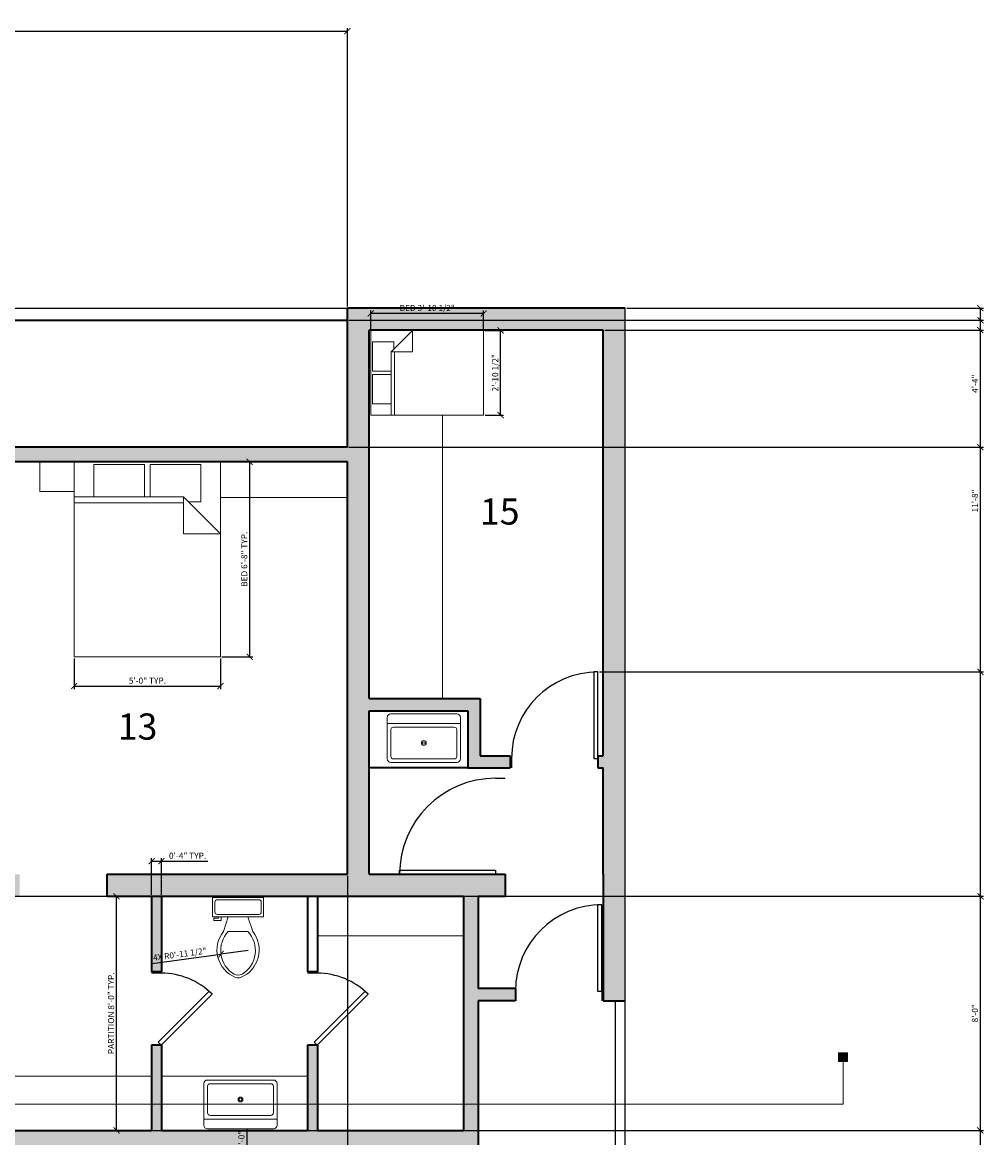
# Model space of a CAD drawing. Units: inches. Extents: x 3122 to 5933, y 1474 to 2995.
# Tile 12 of 12: x 5538 to 5932, y 2536 to 2993. Entities that reach past the tile are written whole.
import ezdxf

# ---------------------------------------------------------------- set-up
doc = ezdxf.new("R2010")
doc.units = ezdxf.units.IN
for name, color, linetype, lineweight in [('A-ANNO-DIMS', 2, 'Continuous', 18), ('A-ANNO-SYMB', 6, 'Continuous', 18), ('A-AREA-IDEN', 7, 'Continuous', 20), ('A-DOOR', 4, 'Continuous', 25), ('A-FLOR-CASE', 8, 'Continuous', 18), ('A-FLOR-FIXT', 9, 'Continuous', 18), ('A-FURN', 8, 'Continuous', 18), ('A-WALL', 7, 'Continuous', 35), ('A-WALL-PATT', 7, 'Continuous', 13), ('C-PROP', 7, 'Continuous', 25)]:
    doc.layers.add(name, color=color, linetype=linetype, lineweight=lineweight)
doc.styles.get("Standard").update_dxf_attribs({"font": 'arial.ttf'})
doc.dimstyles.new('ISO-25', dxfattribs={"dimtxt": 2.5, "dimasz": 2.5, "dimexe": 1.25, "dimexo": 0.625, "dimtad": 1, "dimdec": 0, "dimlunit": 3, "dimtxsty": 'Standard', "dimblk": 'ARCHTICK', "dimcen": 2.5, "dimadec": 0, "dimazin": 0, "dimtfac": 1, "dimtdec": 0, "dimtmove": 0, "dimatfit": 3, "dimfxl": 1, "dimarcsym": 0})

# ---------------------------------------------------------------- blocks, each defined once
blk = doc.blocks.new('*U28')
for p, q in [((0, 0), (0, -100)), ((-900, 0), (-900, -100))]:
    blk.add_line(p, q)
blk.add_lwpolyline([(0, 0), (0, 900), (-43.75, 900), (-43.75, 0)], close=True)
blk.add_arc((0, 0), 900, 90, 180)
blk = doc.blocks.new('*U29')
for p, q in [((0, 0), (0, 100)), ((750, 0), (750, 100))]:
    blk.add_line(p, q)
blk.add_lwpolyline([(0, 0), (530, -530), (561, -499), (31, 31)], close=True)
blk.add_arc((0, 0), 750, 315, 0)
blk = doc.blocks.new('*U30')
for p, q in [((0, 0), (0, -100)), ((1000, 0), (1000, -100))]:
    blk.add_line(p, q)
blk.add_lwpolyline([(0, 0), (0, 1000), (43.75, 1000), (43.75, 0)], close=True)
blk.add_arc((0, 0), 1000, 0, 90)
blk = doc.blocks.new('Bed - Queen')
for p, q in [((0, -80.00003), (0, 0)), ((0, 0), (59.99999, 0)), ((59.99999, 0), (59.99999, -80.00003)), ((7.99999, -1.2), (28.79998, -1.2)), ((7.99999, -14.4), (7.99999, -1.2)), ((28.79998, -1.2), (28.79998, -14.4)), ((31.19999, -1.2), (51.99999, -1.2)), ((31.19999, -14.4), (31.19999, -1.2)), ((51.99999, -1.2), (51.99999, -16.4)), ((0, -14.4), (44.8, -14.4)), ((44.8, -16.8), (0, -16.8)), ((59.99999, -29.6), (44.8, -14.4)), ((44.8, -14.4), (44.8, -29.6)), ((51.99999, -16.4), (46.79936, -16.4)), ((44.8, -29.6), (59.99999, -29.6)), ((59.99999, -80.00003), (0, -80.00003))]:
    blk.add_line(p, q)
blk = doc.blocks.new('Sink-single - 30 in top')
blk.add_line((-15, -3.999996), (15, -3.999996))
for points in [[(-13.5, 0), (13.5, 0)], [(-15, -18.499996), (-15, -1.5)], [(15, -1.5), (15, -18.499996)], [(-13.5, -17.499996), (-13.5, -6.499996)], [(-12.5, -5.499996), (12.5, -5.499996)], [(13.5, -6.499996), (13.5, -17.499996)], [(13.5, -19.999996), (-13.5, -19.999996)], [(12.5, -18.499996), (-12.5, -18.499996)]]:
    blk.add_lwpolyline(points)
for radius in [1, 0.5]:
    blk.add_circle((0, -11.999996), radius)
for centre, radius, start, end in [((-13.5, -1.5), 1.5, 90, 180), ((13.5, -1.5), 1.5, 0, 90), ((-12.5, -6.499996), 1, 90, 180), ((12.5, -6.499996), 1, 0, 90), ((-12.5, -17.499996), 1, 180, 270), ((12.5, -17.499996), 1, 270, 0), ((-13.5, -18.499996), 1.5, 180, 270), ((13.5, -18.499996), 1.5, 270, 0)]:
    blk.add_arc(centre, radius, start, end)
blk = doc.blocks.new('Toilet - top')
for p, q in [((9.5, -6), (9.5, -2)), ((-10, -8.5), (-8, -8.5)), ((-10, -9.5), (-10, -8.5)), ((-8, -8.5), (-8, -8)), ((-7, -8), (-7, -9.5)), ((-4, -8), (-6, -14)), ((4, -8), (6, -14)), ((-7, -9.5), (-10, -9.5)), ((4, -14), (-4, -14))]:
    blk.add_line(p, q)
blk.add_lwpolyline([(10.5, -8), (10.5, 0), (-10.5, 0), (-10.5, -8)], close=True)
for points in [[(-9.5, -2), (-9.5, -6)], [(8.5, -1), (-8.5, -1)], [(-8.5, -7), (8.5, -7)]]:
    blk.add_lwpolyline(points)
for centre, radius, start, end in [((-8.62, -1.88), 0.884, 81.8699, 188.1301), ((8.62, -1.88), 0.884, 351.8699, 98.1301), ((-8.62, -6.12), 0.884, 171.8699, 278.1301), ((8.62, -6.12), 0.884, 261.8699, 8.1301), ((3.52, -21.58), 12.17, 141.4691, 247.9714), ((4.2, -21.82), 11.33, 136.3677, 238.9468), ((-3.52, -21.58), 12.17, 292.0284, 38.5307), ((-4.2, -21.82), 11.33, 301.053, 43.6321), ((0, -27.88), 4, 245.7318, 294.2682), ((0, -29), 4, 254.8605, 285.1395)]:
    blk.add_arc(centre, radius, start, end)
blk = doc.blocks.new('SECTION-LINE-END-MARK')
h = blk.add_hatch(color=256)
h.dxf.hatch_style = 1
h.paths.add_polyline_path([(3.68, 3.54), (0, 3.54), (0, 0), (3.68, 0)])
blk.add_lwpolyline([(0, 3.54), (3.68, 3.54), (3.68, 0), (0, 0)], close=True)
blk = doc.blocks.new('BATH-PARTITION-DOOR-OPENING')
for p, q in [((0, 96), (0, 64.95)), ((4, 96), (4, 64.95)), ((4, 64.95), (0, 64.95)), ((4, 34.95), (0, 34.95)), ((0, 34.95), (0, 0)), ((4, 34.95), (4, 0))]:
    blk.add_line(p, q)
blk = doc.blocks.new('_ArchTick')
at = {"color": 0, "linetype": 'ByBlock', "const_width": 0.15}
blk.add_lwpolyline([(-0.5, -0.5), (0.5, 0.5)], dxfattribs=at)
blk = doc.blocks.new('*D64')
at = {"layer": 'A-ANNO-DIMS', "color": 0, "lineweight": -2, "transparency": 16777216}
for p, q in [((5619.51, 2812.9), (5632.13, 2812.9)), ((5630.88, 2732.9), (5630.88, 2812.9)), ((5619.51, 2732.9), (5632.13, 2732.9))]:
    blk.add_line(p, q, dxfattribs=at)
at = {"layer": 'Defpoints', "color": 0, "transparency": 16777216}
for p in [(5618.88, 2812.9), (5630.88, 2812.9), (5618.88, 2732.9)]:
    blk.add_point(p, dxfattribs=at)
at = {"layer": 'A-ANNO-DIMS', "color": 0, "lineweight": -2, "transparency": 16777216, "xscale": 2.5, "yscale": 2.5, "zscale": 2.5}
for p, rotation in [((5630.88, 2812.9), 90), ((5630.88, 2732.9), 270)]:
    blk.add_blockref('_ArchTick', p, dxfattribs=dict(at, rotation=rotation))
at = {"layer": 'A-ANNO-DIMS', "color": 0, "transparency": 16777216, "insert": (5628.98, 2772.9), "char_height": 2.5, "attachment_point": 5, "rotation": 90}
blk.add_mtext('BED 6\'-8" TYP.', dxfattribs=at)
blk = doc.blocks.new('*D65')
at = {"layer": 'A-ANNO-DIMS', "color": 0, "lineweight": -2, "transparency": 16777216}
for p, q in [((5558.88, 2732.27), (5558.88, 2719.65)), ((5618.88, 2732.27), (5618.88, 2719.65)), ((5558.88, 2720.9), (5618.88, 2720.9))]:
    blk.add_line(p, q, dxfattribs=at)
at = {"layer": 'Defpoints', "color": 0, "transparency": 16777216}
for p in [(5558.88, 2732.9), (5618.88, 2732.9), (5618.88, 2720.9)]:
    blk.add_point(p, dxfattribs=at)
at = {"layer": 'A-ANNO-DIMS', "color": 0, "lineweight": -2, "transparency": 16777216, "xscale": 2.5, "yscale": 2.5, "zscale": 2.5, "rotation": 180}
blk.add_blockref('_ArchTick', (5558.88, 2720.9), dxfattribs=at)
at = {"layer": 'A-ANNO-DIMS', "color": 0, "lineweight": -2, "transparency": 16777216, "xscale": 2.5, "yscale": 2.5, "zscale": 2.5}
blk.add_blockref('_ArchTick', (5618.88, 2720.9), dxfattribs=at)
at = {"layer": 'A-ANNO-DIMS', "color": 0, "transparency": 16777216, "insert": (5588.88, 2722.8), "char_height": 2.5, "attachment_point": 5}
blk.add_mtext('5\'-0" TYP.', dxfattribs=at)
blk = doc.blocks.new('*D66')
at = {"layer": 'A-ANNO-DIMS', "color": 0, "lineweight": -2, "transparency": 16777216}
for p, q in [((5680.57, 2867.39), (5680.57, 2874.97)), ((5726.9, 2873.72), (5680.57, 2873.72)), ((5726.9, 2867.39), (5726.9, 2874.97))]:
    blk.add_line(p, q, dxfattribs=at)
at = {"layer": 'Defpoints', "color": 0, "transparency": 16777216}
for p in [(5680.57, 2873.72), (5680.57, 2866.77), (5726.9, 2866.77)]:
    blk.add_point(p, dxfattribs=at)
at = {"layer": 'A-ANNO-DIMS', "color": 0, "lineweight": -2, "transparency": 16777216, "xscale": 2.5, "yscale": 2.5, "zscale": 2.5, "rotation": 180}
blk.add_blockref('_ArchTick', (5680.57, 2873.72), dxfattribs=at)
at = {"layer": 'A-ANNO-DIMS', "color": 0, "lineweight": -2, "transparency": 16777216, "xscale": 2.5, "yscale": 2.5, "zscale": 2.5}
blk.add_blockref('_ArchTick', (5726.9, 2873.72), dxfattribs=at)
at = {"layer": 'A-ANNO-DIMS', "color": 0, "transparency": 16777216, "insert": (5703.74, 2875.64), "char_height": 2.5, "attachment_point": 5}
blk.add_mtext('BED 3\'-10 1/2"', dxfattribs=at)
blk = doc.blocks.new('*D67')
at = {"layer": 'A-ANNO-DIMS', "color": 0, "lineweight": -2, "transparency": 16777216}
for p, q in [((5727.53, 2866.77), (5735.1, 2866.77)), ((5733.85, 2832.02), (5733.85, 2866.77)), ((5727.53, 2832.02), (5735.1, 2832.02))]:
    blk.add_line(p, q, dxfattribs=at)
at = {"layer": 'Defpoints', "color": 0, "transparency": 16777216}
for p in [(5726.9, 2866.77), (5733.85, 2866.77), (5726.9, 2832.02)]:
    blk.add_point(p, dxfattribs=at)
at = {"layer": 'A-ANNO-DIMS', "color": 0, "lineweight": -2, "transparency": 16777216, "xscale": 2.5, "yscale": 2.5, "zscale": 2.5}
for p, rotation in [((5733.85, 2866.77), 90), ((5733.85, 2832.02), 270)]:
    blk.add_blockref('_ArchTick', p, dxfattribs=dict(at, rotation=rotation))
at = {"layer": 'A-ANNO-DIMS', "color": 0, "transparency": 16777216, "insert": (5731.94, 2849.39), "char_height": 2.5, "attachment_point": 5, "rotation": 90}
blk.add_mtext('2\'-10 1/2"', dxfattribs=at)
blk = doc.blocks.new('*D76')
at = {"layer": 'A-ANNO-DIMS', "color": 0, "lineweight": -2, "transparency": 16777216}
for p, q in [((5590.03, 2634.69), (5575, 2634.69)), ((5576.25, 2538.69), (5576.25, 2634.69)), ((5590.03, 2538.69), (5575, 2538.69))]:
    blk.add_line(p, q, dxfattribs=at)
at = {"layer": 'Defpoints', "color": 0, "transparency": 16777216}
for p in [(5576.25, 2634.69), (5590.65, 2634.69), (5590.65, 2538.69)]:
    blk.add_point(p, dxfattribs=at)
at = {"layer": 'A-ANNO-DIMS', "color": 0, "lineweight": -2, "transparency": 16777216, "xscale": 2.5, "yscale": 2.5, "zscale": 2.5}
for p, rotation in [((5576.25, 2634.69), 90), ((5576.25, 2538.69), 270)]:
    blk.add_blockref('_ArchTick', p, dxfattribs=dict(at, rotation=rotation))
at = {"layer": 'A-ANNO-DIMS', "color": 0, "transparency": 16777216, "insert": (5574.33, 2586.69), "char_height": 2.5, "attachment_point": 5, "rotation": 90}
blk.add_mtext('PARTITION 8\'-0" TYP.', dxfattribs=at)
blk = doc.blocks.new('*D77')
at = {"layer": 'A-ANNO-DIMS', "color": 0, "lineweight": -2, "transparency": 16777216}
for p, q in [((5590.65, 2635.31), (5590.65, 2650.34)), ((5590.65, 2649.09), (5594.65, 2649.09)), ((5594.65, 2635.31), (5594.65, 2650.34)), ((5594.65, 2649.09), (5613.64, 2649.09))]:
    blk.add_line(p, q, dxfattribs=at)
at = {"layer": 'Defpoints', "color": 0, "transparency": 16777216}
for p in [(5594.65, 2649.09), (5590.65, 2634.69), (5594.65, 2634.69)]:
    blk.add_point(p, dxfattribs=at)
at = {"layer": 'A-ANNO-DIMS', "color": 0, "lineweight": -2, "transparency": 16777216, "xscale": 2.5, "yscale": 2.5, "zscale": 2.5, "rotation": 180}
blk.add_blockref('_ArchTick', (5590.65, 2649.09), dxfattribs=at)
at = {"layer": 'A-ANNO-DIMS', "color": 0, "lineweight": -2, "transparency": 16777216, "xscale": 2.5, "yscale": 2.5, "zscale": 2.5}
blk.add_blockref('_ArchTick', (5594.65, 2649.09), dxfattribs=at)
at = {"layer": 'A-ANNO-DIMS', "color": 0, "transparency": 16777216, "insert": (5605.4, 2650.99), "char_height": 2.5, "attachment_point": 5}
blk.add_mtext('0\'-4" TYP.', dxfattribs=at)
blk = doc.blocks.new('*D93')
at = {"layer": 'A-ANNO-DIMS', "color": 0, "lineweight": -2, "transparency": 16777216}
for p, q in [((5785.59, 2875.9), (5931.98, 2875.9)), ((5930.73, 1915.9), (5930.73, 2875.9)), ((5785.59, 1915.9), (5931.98, 1915.9))]:
    blk.add_line(p, q, dxfattribs=at)
at = {"layer": 'Defpoints', "color": 0, "transparency": 16777216}
for p in [(5784.96, 2875.9), (5930.73, 2875.9), (5784.96, 1915.9)]:
    blk.add_point(p, dxfattribs=at)
at = {"layer": 'A-ANNO-DIMS', "color": 0, "lineweight": -2, "transparency": 16777216, "xscale": 2.5, "yscale": 2.5, "zscale": 2.5}
for p, rotation in [((5930.73, 2875.9), 90), ((5930.73, 1915.9), 270)]:
    blk.add_blockref('_ArchTick', p, dxfattribs=dict(at, rotation=rotation))
at = {"layer": 'A-ANNO-DIMS', "color": 0, "transparency": 16777216, "insert": (5928.83, 2395.9), "char_height": 2.5, "attachment_point": 5, "rotation": 90}
blk.add_mtext('80\'-0"', dxfattribs=at)
blk = doc.blocks.new('*D96')
at = {"layer": 'A-ANNO-DIMS', "color": 0, "lineweight": -2, "transparency": 16777216}
for p, q in [((5178.96, 2876.52), (5178.96, 2990.75)), ((5178.96, 2989.5), (5670.96, 2989.5)), ((5670.96, 2876.52), (5670.96, 2990.75))]:
    blk.add_line(p, q, dxfattribs=at)
at = {"layer": 'Defpoints', "color": 0, "transparency": 16777216}
for p in [(5670.96, 2989.5), (5178.96, 2875.9), (5670.96, 2875.9)]:
    blk.add_point(p, dxfattribs=at)
at = {"layer": 'A-ANNO-DIMS', "color": 0, "lineweight": -2, "transparency": 16777216, "xscale": 2.5, "yscale": 2.5, "zscale": 2.5, "rotation": 180}
blk.add_blockref('_ArchTick', (5178.96, 2989.5), dxfattribs=at)
at = {"layer": 'A-ANNO-DIMS', "color": 0, "lineweight": -2, "transparency": 16777216, "xscale": 2.5, "yscale": 2.5, "zscale": 2.5}
blk.add_blockref('_ArchTick', (5670.96, 2989.5), dxfattribs=at)
at = {"layer": 'A-ANNO-DIMS', "color": 0, "transparency": 16777216, "insert": (5424.96, 2991.4), "char_height": 2.5, "attachment_point": 5}
blk.add_mtext('41\'-0"', dxfattribs=at)
blk = doc.blocks.new('*D110')
at = {"layer": 'A-ANNO-DIMS', "color": 0, "lineweight": -2, "transparency": 16777216}
for p, q in [((5487.87, 2643.06), (5487.87, 1792.93)), ((5670.96, 2643.06), (5670.96, 1792.93)), ((5487.87, 1794.18), (5670.96, 1794.18))]:
    blk.add_line(p, q, dxfattribs=at)
at = {"layer": 'Defpoints', "color": 0, "transparency": 16777216}
for p in [(5487.87, 2643.69), (5670.96, 2643.69), (5670.96, 1794.18)]:
    blk.add_point(p, dxfattribs=at)
at = {"layer": 'A-ANNO-DIMS', "color": 0, "lineweight": -2, "transparency": 16777216, "xscale": 2.5, "yscale": 2.5, "zscale": 2.5, "rotation": 180}
blk.add_blockref('_ArchTick', (5487.87, 1794.18), dxfattribs=at)
at = {"layer": 'A-ANNO-DIMS', "color": 0, "lineweight": -2, "transparency": 16777216, "xscale": 2.5, "yscale": 2.5, "zscale": 2.5}
blk.add_blockref('_ArchTick', (5670.96, 1794.18), dxfattribs=at)
at = {"layer": 'A-ANNO-DIMS', "color": 0, "transparency": 16777216, "insert": (5579.42, 1796.09), "char_height": 2.5, "attachment_point": 5}
blk.add_mtext('15\'-3"', dxfattribs=at)
blk = doc.blocks.new('*D111')
at = {"layer": 'A-ANNO-DIMS', "color": 0, "lineweight": -2, "transparency": 16777216}
for p, q in [((5671.588447, 2870.895932), (5931.981923, 2870.895932)), ((5930.731923, 2818.895932), (5930.731923, 2870.895932)), ((5671.588447, 2818.895932), (5931.981923, 2818.895932))]:
    blk.add_line(p, q, dxfattribs=at)
at = {"layer": 'Defpoints', "color": 0, "transparency": 16777216}
for p in [(5670.963447, 2870.895932), (5930.731923, 2870.895932), (5670.963447, 2818.895932)]:
    blk.add_point(p, dxfattribs=at)
at = {"layer": 'A-ANNO-DIMS', "color": 0, "lineweight": -2, "transparency": 16777216, "xscale": 2.5, "yscale": 2.5, "zscale": 2.5}
for p, rotation in [((5930.731923, 2870.895932), 90), ((5930.731923, 2818.895932), 270)]:
    blk.add_blockref('_ArchTick', p, dxfattribs=dict(at, rotation=rotation))
at = {"layer": 'A-ANNO-DIMS', "color": 0, "transparency": 16777216, "insert": (5928.856923, 2844.895932), "char_height": 2.5, "attachment_point": 5, "rotation": 90}
blk.add_mtext('4\'-4"', dxfattribs=at)
blk = doc.blocks.new('*D112')
at = {"layer": 'A-ANNO-DIMS', "color": 0, "lineweight": -2, "transparency": 16777216}
for p, q in [((5776.59, 2866.9), (5931.98, 2866.9)), ((5930.73, 2726.69), (5930.73, 2866.9)), ((5774.41, 2726.69), (5931.98, 2726.69))]:
    blk.add_line(p, q, dxfattribs=at)
at = {"layer": 'Defpoints', "color": 0, "transparency": 16777216}
for p in [(5775.96, 2866.9), (5930.73, 2866.9), (5773.79, 2726.69)]:
    blk.add_point(p, dxfattribs=at)
at = {"layer": 'A-ANNO-DIMS', "color": 0, "lineweight": -2, "transparency": 16777216, "xscale": 2.5, "yscale": 2.5, "zscale": 2.5}
for p, rotation in [((5930.73, 2866.9), 90), ((5930.73, 2726.69), 270)]:
    blk.add_blockref('_ArchTick', p, dxfattribs=dict(at, rotation=rotation))
at = {"layer": 'A-ANNO-DIMS', "color": 0, "transparency": 16777216, "insert": (5928.83, 2796.79), "char_height": 2.5, "attachment_point": 5, "rotation": 90}
blk.add_mtext('11\'-8"', dxfattribs=at)
blk = doc.blocks.new('*D113')
at = {"layer": 'A-ANNO-DIMS', "color": 0, "lineweight": -2, "transparency": 16777216}
for p, q in [((5218.59, 2634.69), (5931.98, 2634.69)), ((5930.73, 2538.69), (5930.73, 2634.69)), ((5218.59, 2538.69), (5931.98, 2538.69))]:
    blk.add_line(p, q, dxfattribs=at)
at = {"layer": 'Defpoints', "color": 0, "transparency": 16777216}
for p in [(5217.96, 2634.69), (5930.73, 2634.69), (5217.96, 2538.69)]:
    blk.add_point(p, dxfattribs=at)
at = {"layer": 'A-ANNO-DIMS', "color": 0, "lineweight": -2, "transparency": 16777216, "xscale": 2.5, "yscale": 2.5, "zscale": 2.5}
for p, rotation in [((5930.73, 2634.69), 90), ((5930.73, 2538.69), 270)]:
    blk.add_blockref('_ArchTick', p, dxfattribs=dict(at, rotation=rotation))
at = {"layer": 'A-ANNO-DIMS', "color": 0, "transparency": 16777216, "insert": (5928.83, 2586.69), "char_height": 2.5, "attachment_point": 5, "rotation": 90}
blk.add_mtext('8\'-0"', dxfattribs=at)
blk = doc.blocks.new('*D129')
at = {"layer": 'A-ANNO-DIMS', "color": 0, "lineweight": -2, "transparency": 16777216}
for p in [(5629.75, 2539.17), (5628.86, 2434.94)]:
    blk.add_line(p, (5629.37, 2495.19), dxfattribs=at)
at = {"layer": 'Defpoints', "color": 0, "transparency": 16777216}
for p in [(5629.37, 2495.19), (5628.86, 2434.94)]:
    blk.add_point(p, dxfattribs=at)
at = {"layer": 'A-ANNO-DIMS', "color": 0, "lineweight": -2, "transparency": 16777216, "xscale": 2.5, "yscale": 2.5, "zscale": 2.5, "rotation": 269.5135960976001}
blk.add_blockref('_ArchTick', (5629.37, 2495.19), dxfattribs=at)
at = {"layer": 'A-ANNO-DIMS', "color": 0, "transparency": 16777216, "insert": (5627.78, 2531.35), "char_height": 2.5, "attachment_point": 5, "rotation": 89.5136}
blk.add_mtext('3X R5\'-0"', dxfattribs=at)
blk = doc.blocks.new('*D132')
at = {"layer": 'A-ANNO-DIMS', "color": 0, "lineweight": -2, "transparency": 16777216}
for p in [(5630.31, 2612.43), (5590.81, 2607.12)]:
    blk.add_line(p, (5619.08, 2610.92), dxfattribs=at)
at = {"layer": 'Defpoints', "color": 0, "transparency": 16777216}
for p in [(5630.31, 2612.43), (5619.08, 2610.92)]:
    blk.add_point(p, dxfattribs=at)
at = {"layer": 'A-ANNO-DIMS', "color": 0, "lineweight": -2, "transparency": 16777216, "xscale": 2.5, "yscale": 2.5, "zscale": 2.5, "rotation": 7.657661803451681}
blk.add_blockref('_ArchTick', (5619.08, 2610.92), dxfattribs=at)
at = {"layer": 'A-ANNO-DIMS', "color": 0, "transparency": 16777216, "insert": (5602.21, 2610.59), "char_height": 2.5, "attachment_point": 5, "rotation": 7.6577}
blk.add_mtext('4X R0\'-11 1/2"', dxfattribs=at)

msp = doc.modelspace()

# ---------------------------------------------------------------- hatches: boundary and pattern name
at = {"layer": 'A-WALL-PATT'}
h = msp.add_hatch(color=256, dxfattribs=at)
h.dxf.hatch_style = 1
h.paths.add_polyline_path([(5536.42, 2643.69), (5487.87, 2643.69), (5487.87, 2667.06), (5485.81, 2667.06), (5481.87, 2667.06), (5481.87, 2643.69), (5481.87, 2590.35), (5487.87, 2590.35), (5487.87, 2634.69), (5524.65, 2634.69), (5524.65, 2538.69), (5487.87, 2538.69), (5487.87, 2554.35), (5481.87, 2554.35), (5481.87, 2532.69), (5524.65, 2532.69), (5658.65, 2532.69), (5718.65, 2532.69), (5718.65, 2501.93), (5724.65, 2501.93), (5724.65, 2549.4), (5718.65, 2549.4), (5718.65, 2538.69), (5658.65, 2538.69), (5658.65, 2573.57), (5658.59, 2573.63), (5654.65, 2573.63), (5654.65, 2538.69), (5594.65, 2538.69), (5594.65, 2573.57), (5594.59, 2573.63), (5590.65, 2573.63), (5590.65, 2538.69), (5530.65, 2538.69), (5530.65, 2634.69), (5536.42, 2634.69)])
h.paths.add_polyline_path([(5735.69, 2643.69), (5679.96, 2643.69), (5679.96, 2710.77), (5720.44, 2710.77), (5720.44, 2687.32), (5737.79, 2687.32), (5737.79, 2692.32), (5725.44, 2692.32), (5725.44, 2715.77), (5679.96, 2715.77), (5679.96, 2866.9), (5775.96, 2866.9), (5775.96, 2692.32), (5773.79, 2692.32), (5773.79, 2687.32), (5775.96, 2687.32), (5775.96, 2643.69), (5775.96, 2591.85), (5784.96, 2591.85), (5784.96, 2875.9), (5670.96, 2875.9), (5670.96, 2818.9), (5412.4, 2818.9), (5412.4, 2812.9), (5460.96, 2812.9), (5460.96, 2719.12), (5404.54, 2719.12), (5404.54, 2713.12), (5466.96, 2713.12), (5481.87, 2713.12), (5481.87, 2703.06), (5487.87, 2703.06), (5487.87, 2719.12), (5466.96, 2719.12), (5466.96, 2812.9), (5670.96, 2812.9), (5670.96, 2643.69), (5572.42, 2643.69), (5572.42, 2634.69), (5718.65, 2634.69), (5718.65, 2549.4), (5724.65, 2549.4), (5724.65, 2591.85), (5739.96, 2591.85), (5739.96, 2596.85), (5724.65, 2596.85), (5724.65, 2634.69), (5735.69, 2634.69)])
h.paths.add_polyline_path([(5594.65, 2634.69), (5590.65, 2634.69), (5590.65, 2603.63), (5594.65, 2603.63)], flags=17)
h.paths.add_polyline_path([(5724.65, 2441.93), (5718.65, 2441.93), (5718.65, 2336.51), (5724.65, 2336.51)])
h.paths.add_polyline_path([(5724.65, 2276.51), (5718.65, 2276.51), (5718.65, 2250.49), (5713.26, 2250.49), (5713.26, 2244.39), (5724.65, 2244.39)])
h.paths.add_polyline_path([(5689.26, 2250.49), (5540.87, 2250.49), (5540.87, 2317.46), (5535.87, 2317.46), (5535.87, 2244.39), (5689.26, 2244.39)])
h.paths.add_polyline_path([(5540.87, 2532.69), (5535.87, 2532.69), (5535.87, 2472.78), (5540.87, 2472.78)])
h.paths.add_polyline_path([(5540.87, 2472.78), (5537.87, 2472.78), (5537.87, 2346.69), (5537.87, 2317.46), (5540.87, 2317.46)])

# ---------------------------------------------------------------- linework, layer by layer
at = {"layer": 'A-ANNO-SYMB'}
for p, q in [((5874.48, 2549.4), (5874.48, 2566.86)), ((5874.48, 2549.4), (4977.78, 2549.4)), ((5658.65, 2549.4), (5784.96, 2549.4)), ((5784.96, 2549.4), (5874.48, 2549.4))]:
    msp.add_line(p, q, dxfattribs=at)
at = {"layer": 'A-FLOR-CASE'}
for p, q in [((5709.98, 2715.77), (5709.98, 2832.02)), ((5618.88, 2798.24), (5670.96, 2798.24))]:
    msp.add_line(p, q, dxfattribs=at)
at = {"layer": 'A-FLOR-FIXT'}
for p, q in [((5718.65, 2618.53), (5658.65, 2618.53)), ((5590.65, 2560.9), (5530.65, 2560.9)), ((5654.65, 2560.9), (5594.65, 2560.9))]:
    msp.add_line(p, q, dxfattribs=at)
at = {"layer": 'A-FURN'}
msp.add_line((5709.98, 2866.77), (5709.98, 2866.9), dxfattribs=at)
msp.add_lwpolyline([(5544.74, 2812.9), (5558.88, 2812.9), (5558.88, 2800.7), (5544.74, 2800.7)], close=True, dxfattribs=at)
at = {"layer": 'A-WALL'}
for p, q in [((5784.96, 2875.9), (5670.96, 2875.9)), ((5670.96, 2818.9), (5670.96, 2875.9)), ((5178.96, 2870.9), (5670.96, 2870.9)), ((5775.96, 2866.9), (5679.96, 2866.9)), ((5679.96, 2715.77), (5679.96, 2866.9)), ((5775.96, 2692.32), (5775.96, 2866.9)), ((5670.96, 2818.9), (5412.4, 2818.9)), ((5670.96, 2812.9), (5466.96, 2812.9)), ((5670.96, 2643.69), (5670.96, 2812.9)), ((5679.96, 2715.77), (5725.44, 2715.77)), ((5725.44, 2715.77), (5725.44, 2692.32)), ((5679.96, 2710.77), (5720.44, 2710.77)), ((5679.96, 2643.69), (5679.96, 2710.77)), ((5720.44, 2710.77), (5720.44, 2687.32)), ((5725.44, 2692.32), (5737.79, 2692.32)), ((5737.79, 2692.32), (5737.79, 2687.32)), ((5773.79, 2692.32), (5773.79, 2687.32)), ((5773.79, 2692.32), (5775.96, 2692.32)), ((5720.44, 2687.32), (5679.96, 2687.32)), ((5720.44, 2687.32), (5737.79, 2687.32)), ((5773.79, 2687.32), (5775.96, 2687.32)), ((5775.96, 2643.69), (5775.96, 2687.32)), ((5572.42, 2643.69), (5670.96, 2643.69)), ((5572.42, 2634.69), (5572.42, 2643.69)), ((5679.96, 2643.69), (5735.69, 2643.69)), ((5735.69, 2643.69), (5735.69, 2634.69)), ((5775.96, 2643.69), (5775.96, 2591.85)), ((5572.42, 2634.69), (5718.65, 2634.69)), ((5718.65, 2634.69), (5718.65, 2538.69)), ((5724.65, 2634.69), (5724.65, 2596.85)), ((5724.65, 2634.69), (5735.69, 2634.69)), ((5739.96, 2596.85), (5724.65, 2596.85)), ((5739.96, 2596.85), (5739.96, 2591.85)), ((5739.96, 2591.85), (5724.65, 2591.85)), ((5724.65, 2591.85), (5724.65, 2244.39)), ((5775.96, 2591.85), (5784.96, 2591.85)), ((5530.65, 2538.69), (5590.65, 2538.69)), ((5594.65, 2538.69), (5654.65, 2538.69)), ((5658.65, 2538.69), (5718.65, 2538.69))]:
    msp.add_line(p, q, dxfattribs=at)
at = {"layer": 'C-PROP'}
for p, q in [((5178.96, 2875.9), (5670.96, 2875.9)), ((5784.96, 1915.9), (5784.96, 2875.9)), ((5780.96, 2256.39), (5780.96, 2591.85))]:
    msp.add_line(p, q, dxfattribs=at)

# ---------------------------------------------------------------- block references
at = {"layer": 'A-ANNO-SYMB'}
msp.add_blockref('SECTION-LINE-END-MARK', (5872.55, 2566.96), dxfattribs=at)
at = {"layer": 'A-DOOR', "xscale": 0.0393700787401575, "yscale": 0.0393700787401575, "zscale": 0.0393700787401575}
for p in [(5773.79, 2691.26), (5775.4, 2595.78)]:
    msp.add_blockref('*U28', p, dxfattribs=at)
at = {"layer": 'A-DOOR', "xscale": 0.0393700787401575, "yscale": 0.0393700787401575, "zscale": 0.0393700787401575, "rotation": 90}
for name, p in [('*U30', (5731.75, 2643.69)), ('*U29', (5594.59, 2573.63)), ('*U29', (5658.59, 2573.63))]:
    msp.add_blockref(name, p, dxfattribs=at)
at = {"layer": 'A-FLOR-FIXT'}
for name, p in [('Sink-single - 30 in top', (5702.35, 2709.54)), ('Toilet - top', (5626.11, 2634.25))]:
    msp.add_blockref(name, p, dxfattribs=at)
at = {"layer": 'A-FLOR-FIXT', "rotation": 180}
msp.add_blockref('Sink-single - 30 in top', (5627.1, 2539.34), dxfattribs=at)
at = {"layer": 'A-FURN', "xscale": 0.5791275342063747, "yscale": 0.5791275342063747, "zscale": 0.5791275342063747, "rotation": 90}
msp.add_blockref('Bed - Queen', (5680.57, 2832.02), dxfattribs=at)
at = {"layer": 'A-FURN'}
msp.add_blockref('Bed - Queen', (5558.88, 2812.9), dxfattribs=at)
at = {"layer": 'A-WALL'}
for p in [(5590.65, 2538.69), (5654.65, 2538.69)]:
    msp.add_blockref('BATH-PARTITION-DOOR-OPENING', p, dxfattribs=at)

# ---------------------------------------------------------------- texts
at = {"layer": 'A-AREA-IDEN'}
for s, p in [('15', (5725.38, 2787.11)), ('13', (5576.76, 2698.93))]:
    msp.add_text(s, height=10.725, rotation=0.0333, dxfattribs=at).set_placement(p)

# ---------------------------------------------------------------- dimensions: what is measured, and where the dimension line sits
at = {"layer": 'A-ANNO-DIMS'}
for base, p1, p2, picture, middle in [((5670.96, 2989.5), (5178.96, 2875.9), (5670.96, 2875.9), '*D96', (5424.96, 2991.4)), ((5670.96, 1794.18), (5487.87, 2643.69), (5670.96, 2643.69), '*D110', (5579.42, 1796.09))]:
    dim = msp.add_linear_dim(base=base, p1=p1, p2=p2, dimstyle='ISO-25', override={"dimdec": 1, "dimlfac": 1, "dimrnd": 0, "dimzin": 1, "dimdsep": 46, "dimlunit": 4, "dimfrac": 2}, dxfattribs=at)
    dim.commit()
    dim.dimension.update_dxf_attribs({"geometry": picture, "text_midpoint": middle})
for base, p1, p2, angle, text, picture, middle in [((5680.57, 2873.72), (5726.9, 2866.77), (5680.57, 2866.77), 180, 'BED <>', '*D66', (5703.74, 2875.64)), ((5630.88, 2812.9), (5618.88, 2732.9), (5618.88, 2812.9), 90, 'BED <> TYP.', '*D64', (5628.98, 2772.9)), ((5576.25, 2634.69), (5590.65, 2538.69), (5590.65, 2634.69), 90, 'PARTITION <> TYP.', '*D76', (5574.33, 2586.69))]:
    dim = msp.add_linear_dim(base=base, p1=p1, p2=p2, angle=angle, text=text, dimstyle='ISO-25', override={"dimdec": 1, "dimlfac": 1, "dimrnd": 0, "dimzin": 1, "dimdsep": 46, "dimlunit": 4, "dimfrac": 2}, dxfattribs=at)
    dim.commit()
    dim.dimension.update_dxf_attribs({"geometry": picture, "text_midpoint": middle})
for base, p1, p2, picture, middle in [((5930.73, 2875.9), (5784.96, 1915.9), (5784.96, 2875.9), '*D93', (5928.83, 2395.9)), ((5930.73, 2870.9), (5670.96, 2818.9), (5670.96, 2870.9), '*D111', (5928.86, 2844.9)), ((5733.8537, 2866.7686), (5726.9041, 2832.021), (5726.9041, 2866.7686), '*D67', (5731.936, 2849.3948)), ((5930.73, 2866.9), (5773.79, 2726.69), (5775.96, 2866.9), '*D112', (5928.83, 2796.79)), ((5930.73, 2634.69), (5217.96, 2538.69), (5217.96, 2634.69), '*D113', (5928.83, 2586.69))]:
    dim = msp.add_linear_dim(base=base, p1=p1, p2=p2, angle=90, dimstyle='ISO-25', override={"dimdec": 1, "dimlfac": 1, "dimrnd": 0, "dimzin": 1, "dimdsep": 46, "dimlunit": 4, "dimfrac": 2}, dxfattribs=at)
    dim.commit()
    dim.dimension.update_dxf_attribs({"geometry": picture, "text_midpoint": middle})
for base, p1, p2, picture, middle in [((5618.88, 2720.9), (5558.88, 2732.9), (5618.88, 2732.9), '*D65', (5588.88, 2722.8)), ((5594.65, 2649.09), (5590.65, 2634.69), (5594.65, 2634.69), '*D77', (5605.4, 2650.99))]:
    dim = msp.add_linear_dim(base=base, p1=p1, p2=p2, text='<> TYP.', dimstyle='ISO-25', override={"dimdec": 1, "dimlfac": 1, "dimrnd": 0, "dimzin": 1, "dimdsep": 46, "dimlunit": 4, "dimfrac": 2}, dxfattribs=at)
    dim.commit()
    dim.dimension.update_dxf_attribs({"geometry": picture, "text_midpoint": middle})
dim = msp.add_radius_dim(center=(5630.31, 2612.43), mpoint=(5619.08, 2610.92), text='4X <>', dimstyle='ISO-25', override={"dimdec": 1, "dimlfac": 1, "dimrnd": 0, "dimzin": 1, "dimdsep": 46, "dimlunit": 4, "dimfrac": 2}, dxfattribs=at)
dim.commit()
dim.dimension.update_dxf_attribs({"geometry": '*D132', "text_midpoint": (5602.21, 2610.59)})
dim = msp.add_radius_dim(center=(5628.8605, 2434.9401), mpoint=(5629.372, 2495.1879), text='3X <>', dimstyle='ISO-25', override={"dimdec": 1, "dimlfac": 1, "dimrnd": 0, "dimzin": 1, "dimdsep": 46, "dimlunit": 4, "dimfrac": 2}, dxfattribs=at)
dim.commit()
dim.dimension.update_dxf_attribs({"geometry": '*D129', "text_midpoint": (5629.6789, 2531.3365), "dimtype": 164})

doc.saveas('drawing.dxf')
